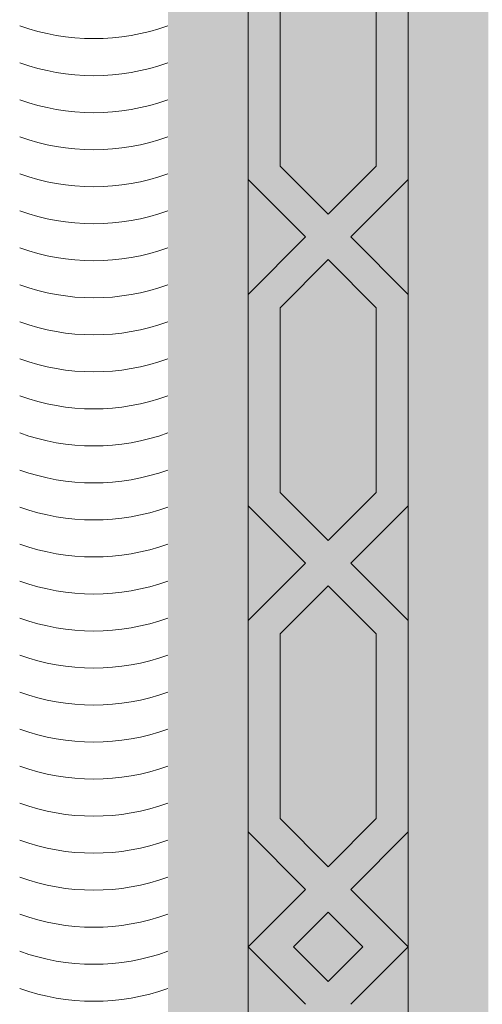
# Model space of a CAD drawing. Units: inches. Extents: x 844 to 2234, y 346 to 1084.
# Tile 30 of 93: x 1249.183 to 1252.862, y 695.763 to 703.597. Entities that reach past the tile are written whole.
import ezdxf

# ---------------------------------------------------------------- set-up
doc = ezdxf.new("R2010")
doc.units = ezdxf.units.IN
doc.header["$MEASUREMENT"] = 0
doc.layers.add('furniture', color=8, linetype='Continuous', lineweight=18)
doc.layers.add('RA-AP-01$0$INT', color=35, linetype='Continuous', lineweight=5)
doc.layers.add('RA-AP-01$0$FURN', color=3, linetype='Continuous')

# ---------------------------------------------------------------- blocks, each defined once
blk = doc.blocks.new('A$C18D01794')
at = {"layer": 'RA-AP-01$0$INT'}
h = blk.add_hatch(color=256, dxfattribs=at)
h.paths.add_polyline_path([(4.35521, -6.15671), (4.35521, -8.05671), (5.45521, -8.05671), (5.45521, -6.15671)])
h.paths.add_polyline_path([(4.40521, -8.00671), (4.40521, -6.20671), (5.40521, -6.20671), (5.40521, -8.00671)], flags=16)
h = blk.add_hatch(color=256, dxfattribs=at)
h.paths.add_polyline_path([(4.46935, -7.07085), (4.50521, -7.035), (4.50521, -7.10671)])
h.paths.add_polyline_path([(4.45521, -7.085), (4.47692, -7.10671), (4.43349, -7.10671)])
h.paths.add_polyline_path([(4.40521, -7.035), (4.44106, -7.07085), (4.40521, -7.10671)])
h.paths.add_polyline_path([(4.42521, -6.91146), (4.45521, -6.88146), (4.48521, -6.91146), (4.48521, -7.02671), (4.45521, -7.05671), (4.42521, -7.02671)])
h.paths.add_polyline_path([(4.50521, -6.83146), (4.50521, -6.90318), (4.46935, -6.86732)])
h.paths.add_polyline_path([(4.42521, -6.70793), (4.45521, -6.67793), (4.48521, -6.70793), (4.48521, -6.82318), (4.45521, -6.85318), (4.42521, -6.82318)])
h.paths.add_polyline_path([(4.42521, -6.50439), (4.45521, -6.47439), (4.48521, -6.50439), (4.48521, -6.61964), (4.45521, -6.64964), (4.42521, -6.61964)])
h.paths.add_polyline_path([(4.46935, -6.66378), (4.50521, -6.62793), (4.50521, -6.69964)])
h.paths.add_polyline_path([(4.40521, -6.62793), (4.44106, -6.66378), (4.40521, -6.69964)])
h.paths.add_polyline_path([(4.40521, -6.42439), (4.44106, -6.46025), (4.40521, -6.49611)])
h.paths.add_polyline_path([(4.46935, -6.46025), (4.50521, -6.42439), (4.50521, -6.49611)])
h.paths.add_polyline_path([(4.42521, -6.30085), (4.45521, -6.27085), (4.48521, -6.30085), (4.48521, -6.41611), (4.45521, -6.44611), (4.42521, -6.41611)])
h.paths.add_polyline_path([(4.42521, -6.22671), (4.47106, -6.22671), (4.42521, -6.27257)])
h.paths.add_polyline_path([(4.49935, -6.22671), (4.63606, -6.22671), (4.66606, -6.25671), (4.63606, -6.28671), (4.49935, -6.28671), (4.46935, -6.25671)])
h.paths.add_polyline_path([(4.68021, -6.27085), (4.71606, -6.30671), (4.64435, -6.30671)])
h.paths.add_polyline_path([(4.64435, -6.20671), (4.71606, -6.20671), (4.68021, -6.24257)])
h.paths.add_polyline_path([(4.72435, -6.22671), (4.86106, -6.22671), (4.89106, -6.25671), (4.86106, -6.28671), (4.72435, -6.28671), (4.69435, -6.25671)])
h.paths.add_polyline_path([(4.90521, -6.27085), (4.94106, -6.30671), (4.86935, -6.30671)])
h.paths.add_polyline_path([(4.86935, -6.20671), (4.94106, -6.20671), (4.90521, -6.24257)])
h.paths.add_polyline_path([(4.94935, -6.22671), (5.08606, -6.22671), (5.11606, -6.25671), (5.08606, -6.28671), (4.94935, -6.28671), (4.91935, -6.25671)])
h.paths.add_polyline_path([(5.13021, -6.27085), (5.16606, -6.30671), (5.09435, -6.30671)])
h.paths.add_polyline_path([(5.09435, -6.20671), (5.16606, -6.20671), (5.13021, -6.24257)])
h.paths.add_polyline_path([(5.17435, -6.22671), (5.31106, -6.22671), (5.34106, -6.25671), (5.31106, -6.28671), (5.17435, -6.28671), (5.14435, -6.25671)])
h.paths.add_polyline_path([(5.32521, -6.30085), (5.35521, -6.27085), (5.38521, -6.30085), (5.38521, -6.41611), (5.35521, -6.44611), (5.32521, -6.41611)])
h.paths.add_polyline_path([(5.33935, -6.22671), (5.38521, -6.22671), (5.38521, -6.27257)])
h.paths.add_polyline_path([(5.32521, -6.50439), (5.35521, -6.47439), (5.38521, -6.50439), (5.38521, -6.61964), (5.35521, -6.64964), (5.32521, -6.61964)])
h.paths.add_polyline_path([(5.30521, -6.42439), (5.34106, -6.46025), (5.30521, -6.49611)])
h.paths.add_polyline_path([(5.36935, -6.46025), (5.40521, -6.42439), (5.40521, -6.49611)])
h.paths.add_polyline_path([(5.40521, -6.62793), (5.40521, -6.69964), (5.36935, -6.66378)])
h.paths.add_polyline_path([(5.30521, -6.62793), (5.34106, -6.66378), (5.30521, -6.69964)])
h.paths.add_polyline_path([(5.32521, -6.70793), (5.35521, -6.67793), (5.38521, -6.70793), (5.38521, -6.82318), (5.35521, -6.85318), (5.32521, -6.82318)])
h.paths.add_polyline_path([(5.30521, -6.83146), (5.34106, -6.86732), (5.30521, -6.90318)])
h.paths.add_polyline_path([(5.32521, -6.91146), (5.35521, -6.88146), (5.38521, -6.91146), (5.38521, -7.02671), (5.35521, -7.05671), (5.32521, -7.02671)])
h.paths.add_polyline_path([(5.40458, -6.83209, 0.001218), (5.40521, -6.83231), (5.40521, -6.90318), (5.36935, -6.86732)])
h.paths.add_polyline_path([(5.36935, -7.07085), (5.40521, -7.035), (5.40521, -7.10671)])
h.paths.add_polyline_path([(5.35521, -7.085), (5.37692, -7.10671), (5.33349, -7.10671)])
h.paths.add_polyline_path([(5.30521, -7.035), (5.34106, -7.07085), (5.30521, -7.10671)])
h = blk.add_hatch(color=256, dxfattribs=at)
h.paths.add_polyline_path([(4.50521, -6.62793), (4.46935, -6.66378), (4.50521, -6.69964), (4.50521, -6.83146), (4.46935, -6.86732), (4.50521, -6.90318), (4.50521, -7.035), (4.46935, -7.07085), (4.50521, -7.10671), (4.47692, -7.10671), (4.45521, -7.085), (4.43349, -7.10671), (4.40521, -7.10671), (4.44106, -7.07085), (4.40521, -7.035), (4.40521, -6.90318), (4.44106, -6.86732), (4.40521, -6.83146), (4.40521, -6.69964), (4.44106, -6.66378), (4.40521, -6.62793), (4.40521, -6.49611), (4.44106, -6.46025), (4.40521, -6.42439), (4.40521, -6.20671), (4.64435, -6.20671), (4.68021, -6.24257), (4.71606, -6.20671), (4.86935, -6.20671), (4.90521, -6.24257), (4.94106, -6.20671), (5.09435, -6.20671), (5.13021, -6.24257), (5.16606, -6.20671), (5.40521, -6.20671), (5.40521, -6.42439), (5.36935, -6.46025), (5.40521, -6.49611), (5.40521, -6.62793), (5.36935, -6.66378), (5.40521, -6.69964), (5.40521, -6.83146), (5.36935, -6.86732), (5.40521, -6.90318), (5.40521, -7.035), (5.36935, -7.07085), (5.40521, -7.10671), (5.37692, -7.10671), (5.35521, -7.085), (5.33349, -7.10671), (5.30521, -7.10671), (5.34106, -7.07085), (5.30521, -7.035), (5.30521, -6.90318), (5.34106, -6.86732), (5.30521, -6.83146), (5.30521, -6.69964), (5.34106, -6.66378), (5.30521, -6.62793), (5.30521, -6.49611), (5.34106, -6.46025), (5.30521, -6.42439), (5.30521, -6.30671), (5.16606, -6.30671), (5.13021, -6.27085), (5.09435, -6.30671), (4.94106, -6.30671), (4.90521, -6.27085), (4.86935, -6.30671), (4.71606, -6.30671), (4.68021, -6.27085), (4.64435, -6.30671), (4.50521, -6.30671), (4.50521, -6.42439), (4.46935, -6.46025), (4.50521, -6.49611)])
h.paths.add_polyline_path([(4.48521, -6.50439), (4.45521, -6.47439), (4.42521, -6.50439), (4.42521, -6.61964), (4.45521, -6.64964), (4.48521, -6.61964)], flags=16)
h.paths.add_polyline_path([(4.45521, -6.44611), (4.48521, -6.41611), (4.48521, -6.30085), (4.45521, -6.27085), (4.42521, -6.30085), (4.42521, -6.41611)], flags=16)
h.paths.add_polyline_path([(4.45521, -6.67793), (4.42521, -6.70793), (4.42521, -6.82318), (4.45521, -6.85318), (4.48521, -6.82318), (4.48521, -6.70793)], flags=16)
h.paths.add_polyline_path([(4.49935, -6.28671), (4.63606, -6.28671), (4.66606, -6.25671), (4.63606, -6.22671), (4.49935, -6.22671), (4.46935, -6.25671)], flags=16)
h.paths.add_polyline_path([(4.42521, -6.27257), (4.47106, -6.22671), (4.42521, -6.22671)], flags=16)
h.paths.add_polyline_path([(4.45521, -6.88146), (4.42521, -6.91146), (4.42521, -7.02671), (4.45521, -7.05671), (4.48521, -7.02671), (4.48521, -6.91146)], flags=16)
h.paths.add_polyline_path([(4.72435, -6.28671), (4.86106, -6.28671), (4.89106, -6.25671), (4.86106, -6.22671), (4.72435, -6.22671), (4.69435, -6.25671)], flags=16)
h.paths.add_polyline_path([(4.91935, -6.25671), (4.94935, -6.28671), (5.08606, -6.28671), (5.11606, -6.25671), (5.08606, -6.22671), (4.94935, -6.22671)], flags=16)
h.paths.add_polyline_path([(5.14435, -6.25671), (5.17435, -6.28671), (5.31106, -6.28671), (5.34106, -6.25671), (5.31106, -6.22671), (5.17435, -6.22671)], flags=16)
h.paths.add_polyline_path([(5.32521, -6.61964), (5.35521, -6.64964), (5.38521, -6.61964), (5.38521, -6.50439), (5.35521, -6.47439), (5.32521, -6.50439)], flags=16)
h.paths.add_polyline_path([(5.32521, -6.41611), (5.35521, -6.44611), (5.38521, -6.41611), (5.38521, -6.30085), (5.35521, -6.27085), (5.32521, -6.30085)], flags=16)
h.paths.add_polyline_path([(5.32521, -6.70793), (5.32521, -6.82318), (5.35521, -6.85318), (5.38521, -6.82318), (5.38521, -6.70793), (5.35521, -6.67793)], flags=16)
h.paths.add_polyline_path([(5.32521, -6.91146), (5.32521, -7.02671), (5.35521, -7.05671), (5.38521, -7.02671), (5.38521, -6.91146), (5.35521, -6.88146)], flags=16)
h.paths.add_polyline_path([(5.33935, -6.22671), (5.38521, -6.27257), (5.38521, -6.22671)], flags=16)
for points in [[(4.50521, -6.30671), (5.30521, -6.30671), (5.30521, -7.10671), (5.25521, -7.10671), (5.25521, -6.35671), (4.55521, -6.35671), (4.55521, -7.10671), (4.50521, -7.10671)], [(4.50521, -7.90671), (5.30521, -7.90671), (5.30521, -7.10671), (5.25521, -7.10671), (5.25521, -7.85671), (4.55521, -7.85671), (4.55521, -7.10671), (4.50521, -7.10671)]]:
    blk.add_hatch(color=256, dxfattribs=at).paths.add_polyline_path(points)
h = blk.add_hatch(color=256, dxfattribs=at)
h.paths.add_polyline_path([(4.50521, -7.5855), (4.46935, -7.54964), (4.50521, -7.51378), (4.50521, -7.38196), (4.46935, -7.34611), (4.50521, -7.31025), (4.50521, -7.17843), (4.46935, -7.14257), (4.50521, -7.10671), (4.47692, -7.10671), (4.45521, -7.12843), (4.43349, -7.10671), (4.40521, -7.10671), (4.44106, -7.14257), (4.40521, -7.17843), (4.40521, -7.31025), (4.44106, -7.34611), (4.40521, -7.38196), (4.40521, -7.51378), (4.44106, -7.54964), (4.40521, -7.5855), (4.40521, -7.71732), (4.44106, -7.75318), (4.40521, -7.78903), (4.40521, -8.00671), (4.64435, -8.00671), (4.68021, -7.97085), (4.71606, -8.00671), (4.86935, -8.00671), (4.90521, -7.97085), (4.94106, -8.00671), (5.09435, -8.00671), (5.13021, -7.97085), (5.16606, -8.00671), (5.40521, -8.00671), (5.40521, -7.78903), (5.36935, -7.75318), (5.40521, -7.71732), (5.40521, -7.5855), (5.36935, -7.54964), (5.40521, -7.51378), (5.40521, -7.38196), (5.36935, -7.34611), (5.40521, -7.31025), (5.40521, -7.17843), (5.36935, -7.14257), (5.40521, -7.10671), (5.37692, -7.10671), (5.35521, -7.12843), (5.33349, -7.10671), (5.30521, -7.10671), (5.34106, -7.14257), (5.30521, -7.17843), (5.30521, -7.31025), (5.34106, -7.34611), (5.30521, -7.38196), (5.30521, -7.51378), (5.34106, -7.54964), (5.30521, -7.5855), (5.30521, -7.71732), (5.34106, -7.75318), (5.30521, -7.78903), (5.30521, -7.90671), (5.16606, -7.90671), (5.13021, -7.94257), (5.09435, -7.90671), (4.94106, -7.90671), (4.90521, -7.94257), (4.86935, -7.90671), (4.71606, -7.90671), (4.68021, -7.94257), (4.64435, -7.90671), (4.50521, -7.90671), (4.50521, -7.78903), (4.46935, -7.75318), (4.50521, -7.71732)])
h.paths.add_polyline_path([(4.48521, -7.70903), (4.45521, -7.73903), (4.42521, -7.70903), (4.42521, -7.59378), (4.45521, -7.56378), (4.48521, -7.59378)], flags=16)
h.paths.add_polyline_path([(4.45521, -7.76732), (4.48521, -7.79732), (4.48521, -7.91257), (4.45521, -7.94257), (4.42521, -7.91257), (4.42521, -7.79732)], flags=16)
h.paths.add_polyline_path([(4.45521, -7.5355), (4.42521, -7.5055), (4.42521, -7.39025), (4.45521, -7.36025), (4.48521, -7.39025), (4.48521, -7.5055)], flags=16)
h.paths.add_polyline_path([(4.49935, -7.92671), (4.63606, -7.92671), (4.66606, -7.95671), (4.63606, -7.98671), (4.49935, -7.98671), (4.46935, -7.95671)], flags=16)
h.paths.add_polyline_path([(4.42521, -7.94085), (4.47106, -7.98671), (4.42521, -7.98671)], flags=16)
h.paths.add_polyline_path([(4.45521, -7.33196), (4.42521, -7.30196), (4.42521, -7.18671), (4.45521, -7.15671), (4.48521, -7.18671), (4.48521, -7.30196)], flags=16)
h.paths.add_polyline_path([(4.72435, -7.92671), (4.86106, -7.92671), (4.89106, -7.95671), (4.86106, -7.98671), (4.72435, -7.98671), (4.69435, -7.95671)], flags=16)
h.paths.add_polyline_path([(4.91935, -7.95671), (4.94935, -7.92671), (5.08606, -7.92671), (5.11606, -7.95671), (5.08606, -7.98671), (4.94935, -7.98671)], flags=16)
h.paths.add_polyline_path([(5.14435, -7.95671), (5.17435, -7.92671), (5.31106, -7.92671), (5.34106, -7.95671), (5.31106, -7.98671), (5.17435, -7.98671)], flags=16)
h.paths.add_polyline_path([(5.32521, -7.59378), (5.35521, -7.56378), (5.38521, -7.59378), (5.38521, -7.70903), (5.35521, -7.73903), (5.32521, -7.70903)], flags=16)
h.paths.add_polyline_path([(5.32521, -7.79732), (5.35521, -7.76732), (5.38521, -7.79732), (5.38521, -7.91257), (5.35521, -7.94257), (5.32521, -7.91257)], flags=16)
h.paths.add_polyline_path([(5.32521, -7.5055), (5.32521, -7.39025), (5.35521, -7.36025), (5.38521, -7.39025), (5.38521, -7.5055), (5.35521, -7.5355)], flags=16)
h.paths.add_polyline_path([(5.32521, -7.30196), (5.32521, -7.18671), (5.35521, -7.15671), (5.38521, -7.18671), (5.38521, -7.30196), (5.35521, -7.33196)], flags=16)
h.paths.add_polyline_path([(5.33935, -7.98671), (5.38521, -7.94085), (5.38521, -7.98671)], flags=16)
h = blk.add_hatch(color=256, dxfattribs=at)
h.paths.add_polyline_path([(4.46935, -7.14257), (4.50521, -7.17843), (4.50521, -7.10671)])
h.paths.add_polyline_path([(4.45521, -7.12843), (4.47692, -7.10671), (4.43349, -7.10671)])
h.paths.add_polyline_path([(4.40521, -7.17843), (4.44106, -7.14257), (4.40521, -7.10671)])
h.paths.add_polyline_path([(4.42521, -7.30196), (4.45521, -7.33196), (4.48521, -7.30196), (4.48521, -7.18671), (4.45521, -7.15671), (4.42521, -7.18671)])
h.paths.add_polyline_path([(4.50521, -7.38196), (4.50521, -7.31025), (4.46935, -7.34611)])
h.paths.add_polyline_path([(4.42521, -7.5055), (4.45521, -7.5355), (4.48521, -7.5055), (4.48521, -7.39025), (4.45521, -7.36025), (4.42521, -7.39025)])
h.paths.add_polyline_path([(4.42521, -7.70903), (4.45521, -7.73903), (4.48521, -7.70903), (4.48521, -7.59378), (4.45521, -7.56378), (4.42521, -7.59378)])
h.paths.add_polyline_path([(4.46935, -7.54964), (4.50521, -7.5855), (4.50521, -7.51378)])
h.paths.add_polyline_path([(4.40521, -7.5855), (4.44106, -7.54964), (4.40521, -7.51378)])
h.paths.add_polyline_path([(4.40521, -7.78903), (4.44106, -7.75318), (4.40521, -7.71732)])
h.paths.add_polyline_path([(4.46935, -7.75318), (4.50521, -7.78903), (4.50521, -7.71732)])
h.paths.add_polyline_path([(4.42521, -7.91257), (4.45521, -7.94257), (4.48521, -7.91257), (4.48521, -7.79732), (4.45521, -7.76732), (4.42521, -7.79732)])
h.paths.add_polyline_path([(4.42521, -7.98671), (4.47106, -7.98671), (4.42521, -7.94085)])
h.paths.add_polyline_path([(4.49935, -7.98671), (4.63606, -7.98671), (4.66606, -7.95671), (4.63606, -7.92671), (4.49935, -7.92671), (4.46935, -7.95671)])
h.paths.add_polyline_path([(4.68021, -7.94257), (4.71606, -7.90671), (4.64435, -7.90671)])
h.paths.add_polyline_path([(4.64435, -8.00671), (4.71606, -8.00671), (4.68021, -7.97085)])
h.paths.add_polyline_path([(4.72435, -7.98671), (4.86106, -7.98671), (4.89106, -7.95671), (4.86106, -7.92671), (4.72435, -7.92671), (4.69435, -7.95671)])
h.paths.add_polyline_path([(4.90521, -7.94257), (4.94106, -7.90671), (4.86935, -7.90671)])
h.paths.add_polyline_path([(4.86935, -8.00671), (4.94106, -8.00671), (4.90521, -7.97085)])
h.paths.add_polyline_path([(4.94935, -7.98671), (5.08606, -7.98671), (5.11606, -7.95671), (5.08606, -7.92671), (4.94935, -7.92671), (4.91935, -7.95671)])
h.paths.add_polyline_path([(5.13021, -7.94257), (5.16606, -7.90671), (5.09435, -7.90671)])
h.paths.add_polyline_path([(5.09435, -8.00671), (5.16606, -8.00671), (5.13021, -7.97085)])
h.paths.add_polyline_path([(5.17435, -7.98671), (5.31106, -7.98671), (5.34106, -7.95671), (5.31106, -7.92671), (5.17435, -7.92671), (5.14435, -7.95671)])
h.paths.add_polyline_path([(5.32521, -7.91257), (5.35521, -7.94257), (5.38521, -7.91257), (5.38521, -7.79732), (5.35521, -7.76732), (5.32521, -7.79732)])
h.paths.add_polyline_path([(5.33935, -7.98671), (5.38521, -7.98671), (5.38521, -7.94085)])
h.paths.add_polyline_path([(5.32521, -7.70903), (5.35521, -7.73903), (5.38521, -7.70903), (5.38521, -7.59378), (5.35521, -7.56378), (5.32521, -7.59378)])
h.paths.add_polyline_path([(5.30521, -7.78903), (5.34106, -7.75318), (5.30521, -7.71732)])
h.paths.add_polyline_path([(5.36935, -7.75318), (5.40521, -7.78903), (5.40521, -7.71732)])
h.paths.add_polyline_path([(5.40521, -7.5855), (5.40521, -7.51378), (5.36935, -7.54964)])
h.paths.add_polyline_path([(5.30521, -7.5855), (5.34106, -7.54964), (5.30521, -7.51378)])
h.paths.add_polyline_path([(5.32521, -7.5055), (5.35521, -7.5355), (5.38521, -7.5055), (5.38521, -7.39025), (5.35521, -7.36025), (5.32521, -7.39025)])
h.paths.add_polyline_path([(5.30521, -7.38196), (5.34106, -7.34611), (5.30521, -7.31025)])
h.paths.add_polyline_path([(5.32521, -7.30196), (5.35521, -7.33196), (5.38521, -7.30196), (5.38521, -7.18671), (5.35521, -7.15671), (5.32521, -7.18671)])
h.paths.add_polyline_path([(5.40458, -7.38134, -0.001218), (5.40521, -7.38111), (5.40521, -7.31025), (5.36935, -7.34611)])
h.paths.add_polyline_path([(5.36935, -7.14257), (5.40521, -7.17843), (5.40521, -7.10671)])
h.paths.add_polyline_path([(5.35521, -7.12843), (5.37692, -7.10671), (5.33349, -7.10671)])
h.paths.add_polyline_path([(5.30521, -7.17843), (5.34106, -7.14257), (5.30521, -7.10671)])
for p, q in [((5.34106, -7.07085), (5.30521, -7.10671)), ((5.36935, -7.07085), (5.40521, -7.10671)), ((5.35521, -7.085), (5.33349, -7.10671)), ((5.35521, -7.085), (5.37692, -7.10671)), ((5.34106, -7.14257), (5.30521, -7.10671)), ((5.35521, -7.12843), (5.33349, -7.10671)), ((5.35521, -7.12843), (5.37692, -7.10671)), ((5.36935, -7.14257), (5.40521, -7.10671)), ((5.30521, -7.17843), (5.34106, -7.14257)), ((5.40521, -7.17843), (5.36935, -7.14257)), ((5.32521, -7.18671), (5.35521, -7.15671)), ((5.38521, -7.18671), (5.35521, -7.15671)), ((5.32521, -7.30196), (5.32521, -7.18671)), ((5.38521, -7.30196), (5.38521, -7.18671)), ((5.32521, -7.30196), (5.35521, -7.33196)), ((5.38521, -7.30196), (5.35521, -7.33196)), ((5.30521, -7.31025), (5.34106, -7.34611)), ((5.40521, -7.31025), (5.36935, -7.34611)), ((5.30521, -7.38196), (5.34106, -7.34611)), ((5.40521, -7.38196), (5.36935, -7.34611)), ((5.32521, -7.39025), (5.35521, -7.36025)), ((5.38521, -7.39025), (5.35521, -7.36025)), ((5.32521, -7.39025), (5.32521, -7.5055)), ((5.38521, -7.39025), (5.38521, -7.5055)), ((5.32521, -7.5055), (5.35521, -7.5355)), ((5.38521, -7.5055), (5.35521, -7.5355)), ((5.30521, -7.51378), (5.34106, -7.54964)), ((5.40521, -7.51378), (5.36935, -7.54964)), ((5.30521, -7.5855), (5.34106, -7.54964)), ((5.40521, -7.5855), (5.36935, -7.54964)), ((5.32521, -7.59378), (5.35521, -7.56378)), ((5.38521, -7.59378), (5.35521, -7.56378)), ((5.32521, -7.59378), (5.32521, -7.70903)), ((5.38521, -7.59378), (5.38521, -7.70903))]:
    blk.add_line(p, q, dxfattribs=at)
for points in [[(5.40521, -7.10671), (5.40521, -6.20671)], [(5.30521, -7.10671), (5.30521, -6.30671), (4.50521, -6.30671), (4.50521, -7.10671)], [(5.30521, -7.10671), (5.30521, -7.90671), (4.50521, -7.90671), (4.50521, -7.10671)], [(5.40521, -7.10671), (5.40521, -8.00671)]]:
    blk.add_lwpolyline(points, dxfattribs=at)
for centre in [(5.50141, -7.20916), (5.50141, -7.23226), (5.50141, -7.25536), (5.50141, -7.27846), (5.50141, -7.30156), (5.50141, -7.32466), (5.50141, -7.34776), (5.50141, -7.37086), (5.50141, -7.39396), (5.50141, -7.41706), (5.50141, -7.44016), (5.50141, -7.46326), (5.50141, -7.48636), (5.50141, -7.50946), (5.50141, -7.53256), (5.50141, -7.55566), (5.50141, -7.57876), (5.50141, -7.60186), (5.50141, -7.62496), (5.50141, -7.64806), (5.50141, -7.67116), (5.50141, -7.67116), (5.50141, -7.69426), (5.50141, -7.71736), (5.50141, -7.74046), (5.50141, -7.76356), (5.50141, -7.78666), (5.50141, -7.80976)]:
    blk.add_arc(centre, 0.13641, 70.20384, 109.79616, dxfattribs=at)
blk = doc.blocks.new('A$C5D2F253E')
at = {"layer": 'RA-AP-01$0$FURN', "xscale": -0.7999999999883585, "yscale": 0.7999999999883585, "zscale": 0.8, "rotation": 90}
blk.add_blockref('A$C18D01794', (-5.68776, 4.75792), dxfattribs=at)

msp = doc.modelspace()

# ---------------------------------------------------------------- block references
at = {"layer": 'furniture', "xscale": -15.94108302203742, "yscale": 15.94108302203742, "zscale": 15.94108302203742, "rotation": 270}
msp.add_blockref('A$C5D2F253E', (1244.0841, 696.2585), dxfattribs=at)

doc.saveas('drawing.dxf')
